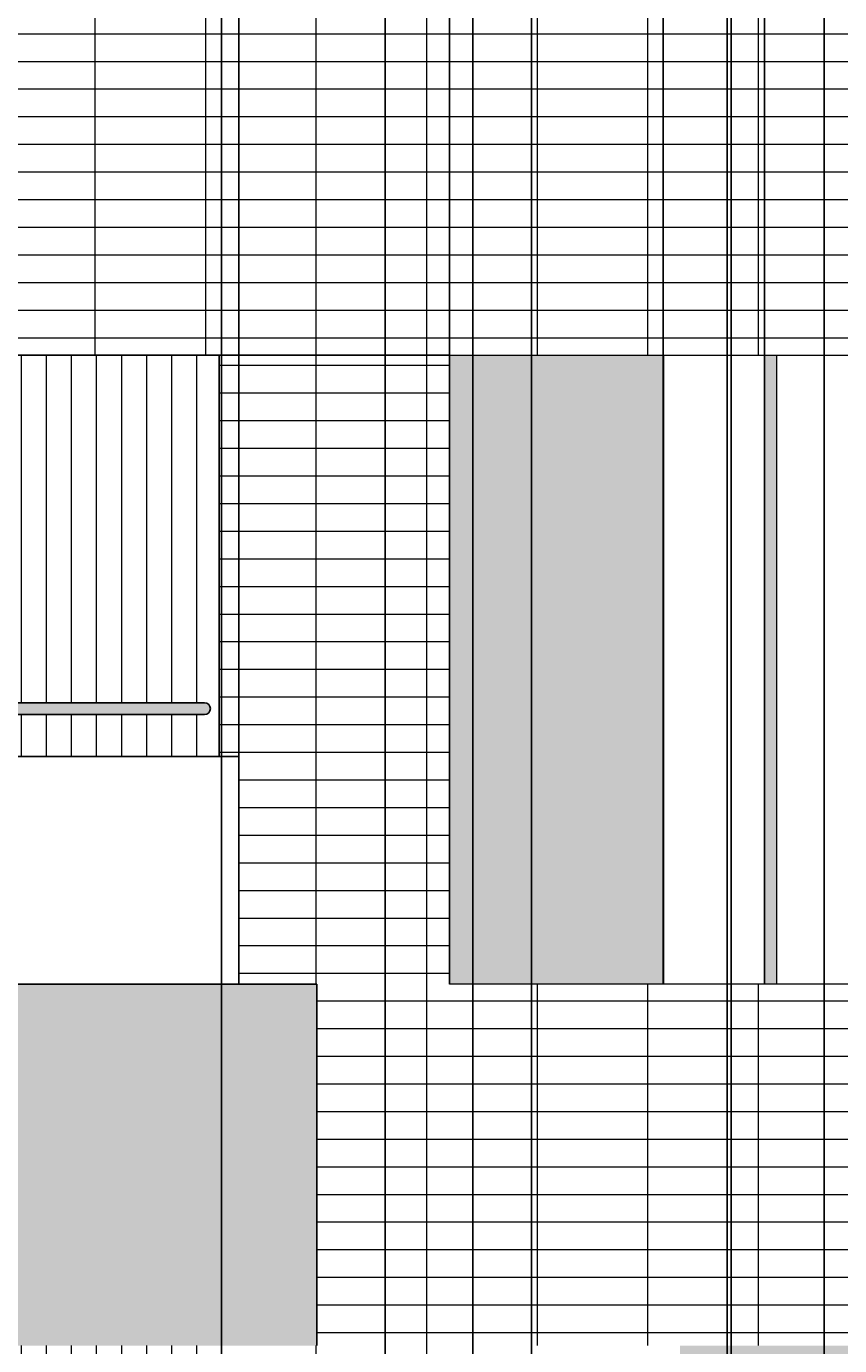
# Model space of a CAD drawing. Units: inches. Extents: x 241 to 943, y 109 to 1396.
# Tile 26 of 34: x 532 to 670, y 842 to 1065. Entities that reach past the tile are written whole.
import ezdxf

# ---------------------------------------------------------------- set-up
doc = ezdxf.new("R2010")
doc.units = ezdxf.units.IN
doc.header["$MEASUREMENT"] = 0
for name, color, linetype, lineweight in [('A-ANNO-DIMS', 2, 'Continuous', 18), ('A-ELEV', 7, 'Continuous', 25), ('A-ELEV-SHAD', 9, 'Continuous', 13), ('A-GLAZ', 4, 'Continuous', 18), ('A-GLAZ-PATT', 18, 'Continuous', 13), ('A-WALL-PATT', 8, 'Continuous', 13)]:
    doc.layers.add(name, color=color, linetype=linetype, lineweight=lineweight)
doc.styles.get("Standard").update_dxf_attribs({"font": 'arial.ttf'})
doc.dimstyles.get("Standard").update_dxf_attribs({"dimtxt": 1.4375, "dimasz": 0.18, "dimexe": 0.18, "dimexo": 0.0625, "dimgap": 0.09, "dimtad": 0, "dimtih": 1, "dimtoh": 1, "dimdec": 4, "dimzin": 0, "dimdsep": 46, "dimlunit": 4, "dimtxsty": 'Standard', "dimcen": 0.09, "dimadec": 0, "dimazin": 0, "dimtfac": 1, "dimtdec": 4, "dimtofl": 0, "dimtmove": 0, "dimatfit": 3, "dimfxl": 1, "dimtolj": 1, "dimtzin": 0, "dimarcsym": 0})

# ---------------------------------------------------------------- blocks, each defined once
blk = doc.blocks.new('*D12')
at = {"layer": 'A-ANNO-DIMS', "color": 0, "lineweight": -2, "transparency": 16777216}
for p, q in [((530.23, 384.24), (530.23, 1395.05)), ((530.41, 1394.87), (587.56, 1394.87)), ((650.73, 1394.87), (593.58, 1394.87)), ((650.91, 384.24), (650.91, 1395.05))]:
    blk.add_line(p, q, dxfattribs=at)
at = {"layer": 'A-ANNO-DIMS', "color": 0, "transparency": 16777216}
for points in [[(530.41, 1394.9), (530.41, 1394.84), (530.23, 1394.87)], [(650.73, 1394.9), (650.73, 1394.84), (650.91, 1394.87)]]:
    blk.add_solid(points, dxfattribs=at)
at = {"layer": 'Defpoints', "color": 0, "transparency": 16777216}
for p in [(650.91, 1394.87), (530.23, 384.18), (650.91, 384.18)]:
    blk.add_point(p, dxfattribs=at)
at = {"layer": 'A-ANNO-DIMS', "color": 0, "transparency": 16777216, "insert": (590.57, 1394.87), "char_height": 1.438, "attachment_point": 5}
blk.add_mtext('\\A1;120.68', dxfattribs=at)
blk = doc.blocks.new('*D13')
at = {"layer": 'A-ANNO-DIMS', "color": 0, "lineweight": -2, "transparency": 16777216}
for p, q in [((650.91, 384.24), (650.91, 1395.05)), ((651.09, 1394.87), (656.14, 1394.87)), ((667.21, 1394.87), (662.16, 1394.87)), ((667.39, 290.06), (667.39, 1395.05))]:
    blk.add_line(p, q, dxfattribs=at)
at = {"layer": 'A-ANNO-DIMS', "color": 0, "transparency": 16777216}
for points in [[(651.09, 1394.9), (651.09, 1394.84), (650.91, 1394.87)], [(667.21, 1394.9), (667.21, 1394.84), (667.39, 1394.87)]]:
    blk.add_solid(points, dxfattribs=at)
at = {"layer": 'Defpoints', "color": 0, "transparency": 16777216}
for p in [(667.39, 1394.87), (650.91, 384.18), (667.39, 290)]:
    blk.add_point(p, dxfattribs=at)
at = {"layer": 'A-ANNO-DIMS', "color": 0, "transparency": 16777216, "insert": (659.15, 1394.87), "char_height": 1.438, "attachment_point": 5}
blk.add_mtext('\\A1;16.486', dxfattribs=at)
blk = doc.blocks.new('*D14')
at = {"layer": 'A-ANNO-DIMS', "color": 0, "lineweight": -2, "transparency": 16777216}
for p, q in [((667.39, 290.06), (667.39, 1395.05)), ((667.57, 1394.87), (727.7, 1394.87)), ((793.85, 1394.87), (733.72, 1394.87)), ((794.03, 290.06), (794.03, 1395.05))]:
    blk.add_line(p, q, dxfattribs=at)
at = {"layer": 'A-ANNO-DIMS', "color": 0, "transparency": 16777216}
for points in [[(667.57, 1394.9), (667.57, 1394.84), (667.39, 1394.87)], [(793.85, 1394.9), (793.85, 1394.84), (794.03, 1394.87)]]:
    blk.add_solid(points, dxfattribs=at)
at = {"layer": 'Defpoints', "color": 0, "transparency": 16777216}
for p in [(794.03, 1394.87), (667.39, 290), (794.03, 290)]:
    blk.add_point(p, dxfattribs=at)
at = {"layer": 'A-ANNO-DIMS', "color": 0, "transparency": 16777216, "insert": (730.71, 1394.87), "char_height": 1.438, "attachment_point": 5}
blk.add_mtext('\\A1;126.63', dxfattribs=at)
blk = doc.blocks.new('*D62')
at = {"layer": 'A-ANNO-DIMS', "color": 0, "lineweight": -2, "transparency": 16777216}
for p, q in [((424.11, 568.89), (424.11, 1395.05)), ((424.29, 1394.87), (492.35, 1394.87)), ((565.02, 1394.87), (496.96, 1394.87)), ((565.2, 568.89), (565.2, 1395.05))]:
    blk.add_line(p, q, dxfattribs=at)
at = {"layer": 'A-ANNO-DIMS', "color": 0, "transparency": 16777216}
for points in [[(424.29, 1394.9), (424.29, 1394.84), (424.11, 1394.87)], [(565.02, 1394.9), (565.02, 1394.84), (565.2, 1394.87)]]:
    blk.add_solid(points, dxfattribs=at)
at = {"layer": 'Defpoints', "color": 0, "transparency": 16777216}
for p in [(565.2, 1394.87), (424.11, 568.83), (565.2, 568.83)]:
    blk.add_point(p, dxfattribs=at)
at = {"layer": 'A-ANNO-DIMS', "color": 0, "transparency": 16777216, "insert": (494.66, 1394.87), "char_height": 1.438, "attachment_point": 5}
blk.add_mtext('\\A1;141.1', dxfattribs=at)
blk = doc.blocks.new('*D63')
at = {"layer": 'A-ANNO-DIMS', "color": 0, "lineweight": -2, "transparency": 16777216}
for p, q in [((651.6, 568.89), (651.6, 1395.05)), ((651.78, 1394.87), (719.84, 1394.87)), ((792.51, 1394.87), (724.45, 1394.87)), ((792.69, 568.89), (792.69, 1395.05))]:
    blk.add_line(p, q, dxfattribs=at)
at = {"layer": 'A-ANNO-DIMS', "color": 0, "transparency": 16777216}
for points in [[(651.78, 1394.9), (651.78, 1394.84), (651.6, 1394.87)], [(792.51, 1394.9), (792.51, 1394.84), (792.69, 1394.87)]]:
    blk.add_solid(points, dxfattribs=at)
at = {"layer": 'Defpoints', "color": 0, "transparency": 16777216}
for p in [(792.69, 1394.87), (651.6, 568.83), (792.69, 568.83)]:
    blk.add_point(p, dxfattribs=at)
at = {"layer": 'A-ANNO-DIMS', "color": 0, "transparency": 16777216, "insert": (722.14, 1394.87), "char_height": 1.438, "attachment_point": 5}
blk.add_mtext('\\A1;141.1', dxfattribs=at)
blk = doc.blocks.new('*D65')
at = {"layer": 'A-ANNO-DIMS', "color": 0, "lineweight": -2, "transparency": 16777216}
for p, q in [((424.11, 700.85), (424.11, 1395.05)), ((424.29, 1394.87), (505.52, 1394.87)), ((592.77, 1394.87), (511.54, 1394.87)), ((592.95, 700.85), (592.95, 1395.05))]:
    blk.add_line(p, q, dxfattribs=at)
at = {"layer": 'A-ANNO-DIMS', "color": 0, "transparency": 16777216}
for points in [[(424.29, 1394.9), (424.29, 1394.84), (424.11, 1394.87)], [(592.77, 1394.9), (592.77, 1394.84), (592.95, 1394.87)]]:
    blk.add_solid(points, dxfattribs=at)
at = {"layer": 'Defpoints', "color": 0, "transparency": 16777216}
for p in [(592.95, 1394.87), (424.11, 700.79), (592.95, 700.79)]:
    blk.add_point(p, dxfattribs=at)
at = {"layer": 'A-ANNO-DIMS', "color": 0, "transparency": 16777216, "insert": (508.53, 1394.87), "char_height": 1.438, "attachment_point": 5}
blk.add_mtext('\\A1;168.85', dxfattribs=at)
blk = doc.blocks.new('*D66')
at = {"layer": 'A-ANNO-DIMS', "color": 0, "lineweight": -2, "transparency": 16777216}
for p, q in [((617.76, 702.85), (617.76, 1395.05)), ((617.94, 1394.87), (680.69, 1394.87)), ((749.45, 1394.87), (686.7, 1394.87)), ((749.63, 702.85), (749.63, 1395.05))]:
    blk.add_line(p, q, dxfattribs=at)
at = {"layer": 'A-ANNO-DIMS', "color": 0, "transparency": 16777216}
for points in [[(617.94, 1394.9), (617.94, 1394.84), (617.76, 1394.87)], [(749.45, 1394.9), (749.45, 1394.84), (749.63, 1394.87)]]:
    blk.add_solid(points, dxfattribs=at)
at = {"layer": 'Defpoints', "color": 0, "transparency": 16777216}
for p in [(749.63, 1394.87), (617.76, 702.79), (749.63, 702.79)]:
    blk.add_point(p, dxfattribs=at)
at = {"layer": 'A-ANNO-DIMS', "color": 0, "transparency": 16777216, "insert": (683.7, 1394.87), "char_height": 1.438, "attachment_point": 5}
blk.add_mtext('\\A1;131.87', dxfattribs=at)
blk = doc.blocks.new('*D67')
at = {"layer": 'A-ANNO-DIMS', "color": 0, "lineweight": -2, "transparency": 16777216}
for p, q in [((389.04, 773.55), (389.04, 1395.05)), ((389.22, 1394.87), (495.34, 1394.87)), ((607.64, 1394.87), (501.52, 1394.87)), ((607.82, 773.55), (607.82, 1395.05))]:
    blk.add_line(p, q, dxfattribs=at)
at = {"layer": 'A-ANNO-DIMS', "color": 0, "transparency": 16777216}
for points in [[(389.22, 1394.9), (389.22, 1394.84), (389.04, 1394.87)], [(607.64, 1394.9), (607.64, 1394.84), (607.82, 1394.87)]]:
    blk.add_solid(points, dxfattribs=at)
at = {"layer": 'Defpoints', "color": 0, "transparency": 16777216}
for p in [(607.82, 1394.87), (389.04, 773.49), (607.82, 773.49)]:
    blk.add_point(p, dxfattribs=at)
at = {"layer": 'A-ANNO-DIMS', "color": 0, "transparency": 16777216, "insert": (498.43, 1394.87), "char_height": 1.438, "attachment_point": 5}
blk.add_mtext('\\A1;218.77', dxfattribs=at)
blk = doc.blocks.new('*D68')
at = {"layer": 'A-ANNO-DIMS', "color": 0, "lineweight": -2, "transparency": 16777216}
for p, q in [((617.76, 841.6), (617.76, 1395.05)), ((617.94, 1394.87), (702.22, 1394.87)), ((792.51, 1394.87), (708.23, 1394.87)), ((792.69, 841.6), (792.69, 1395.05))]:
    blk.add_line(p, q, dxfattribs=at)
at = {"layer": 'A-ANNO-DIMS', "color": 0, "transparency": 16777216}
for points in [[(617.94, 1394.9), (617.94, 1394.84), (617.76, 1394.87)], [(792.51, 1394.9), (792.51, 1394.84), (792.69, 1394.87)]]:
    blk.add_solid(points, dxfattribs=at)
at = {"layer": 'Defpoints', "color": 0, "transparency": 16777216}
for p in [(792.69, 1394.87), (617.76, 841.54), (792.69, 841.54)]:
    blk.add_point(p, dxfattribs=at)
at = {"layer": 'A-ANNO-DIMS', "color": 0, "transparency": 16777216, "insert": (705.23, 1394.87), "char_height": 1.438, "attachment_point": 5}
blk.add_mtext('\\A1;174.93', dxfattribs=at)
blk = doc.blocks.new('*D69')
at = {"layer": 'A-ANNO-DIMS', "color": 0, "lineweight": -2, "transparency": 16777216}
for p, q in [((389.04, 941.55), (389.04, 1395.05)), ((389.22, 1394.87), (476.28, 1394.87)), ((567.95, 1394.87), (480.9, 1394.87)), ((568.13, 941.55), (568.13, 1395.05))]:
    blk.add_line(p, q, dxfattribs=at)
at = {"layer": 'A-ANNO-DIMS', "color": 0, "transparency": 16777216}
for points in [[(389.22, 1394.9), (389.22, 1394.84), (389.04, 1394.87)], [(567.95, 1394.9), (567.95, 1394.84), (568.13, 1394.87)]]:
    blk.add_solid(points, dxfattribs=at)
at = {"layer": 'Defpoints', "color": 0, "transparency": 16777216}
for p in [(568.13, 1394.87), (389.04, 941.49), (568.13, 941.49)]:
    blk.add_point(p, dxfattribs=at)
at = {"layer": 'A-ANNO-DIMS', "color": 0, "transparency": 16777216, "insert": (478.59, 1394.87), "char_height": 1.438, "attachment_point": 5}
blk.add_mtext('\\A1;179.1', dxfattribs=at)
blk = doc.blocks.new('*D70')
at = {"layer": 'A-ANNO-DIMS', "color": 0, "lineweight": -2, "transparency": 16777216}
for p, q in [((603.87, 1009.6), (603.87, 1395.05)), ((604.05, 1394.87), (674.69, 1394.87)), ((751.33, 1394.87), (680.69, 1394.87)), ((751.51, 1009.6), (751.51, 1395.05))]:
    blk.add_line(p, q, dxfattribs=at)
at = {"layer": 'A-ANNO-DIMS', "color": 0, "transparency": 16777216}
for points in [[(604.05, 1394.9), (604.05, 1394.84), (603.87, 1394.87)], [(751.33, 1394.9), (751.33, 1394.84), (751.51, 1394.87)]]:
    blk.add_solid(points, dxfattribs=at)
at = {"layer": 'Defpoints', "color": 0, "transparency": 16777216}
for p in [(751.51, 1394.87), (603.87, 1009.54), (751.51, 1009.54)]:
    blk.add_point(p, dxfattribs=at)
at = {"layer": 'A-ANNO-DIMS', "color": 0, "transparency": 16777216, "insert": (677.69, 1394.87), "char_height": 1.438, "attachment_point": 5}
blk.add_mtext('\\A1;147.64', dxfattribs=at)
blk = doc.blocks.new('*D82')
at = {"layer": 'A-ANNO-DIMS', "color": 0, "lineweight": -2, "transparency": 16777216}
for p, q in [((565.2, 568.89), (565.2, 1395.05)), ((565.38, 1394.87), (605.89, 1394.87)), ((651.42, 1394.87), (610.91, 1394.87)), ((651.6, 568.89), (651.6, 1395.05))]:
    blk.add_line(p, q, dxfattribs=at)
at = {"layer": 'A-ANNO-DIMS', "color": 0, "transparency": 16777216}
for points in [[(565.38, 1394.9), (565.38, 1394.84), (565.2, 1394.87)], [(651.42, 1394.9), (651.42, 1394.84), (651.6, 1394.87)]]:
    blk.add_solid(points, dxfattribs=at)
at = {"layer": 'Defpoints', "color": 0, "transparency": 16777216}
for p in [(651.6, 1394.87), (565.2, 568.83), (651.6, 568.83)]:
    blk.add_point(p, dxfattribs=at)
at = {"layer": 'A-ANNO-DIMS', "color": 0, "transparency": 16777216, "insert": (608.4, 1394.87), "char_height": 1.438, "attachment_point": 5}
blk.add_mtext('\\A1;86.40', dxfattribs=at)
blk = doc.blocks.new('*D83')
at = {"layer": 'A-ANNO-DIMS', "color": 0, "lineweight": -2, "transparency": 16777216}
for p, q in [((592.95, 700.85), (592.95, 1395.05)), ((593.13, 1394.87), (602.27, 1394.87)), ((617.58, 1394.87), (608.45, 1394.87)), ((617.76, 702.85), (617.76, 1395.05))]:
    blk.add_line(p, q, dxfattribs=at)
at = {"layer": 'A-ANNO-DIMS', "color": 0, "transparency": 16777216}
for points in [[(593.13, 1394.9), (593.13, 1394.84), (592.95, 1394.87)], [(617.58, 1394.9), (617.58, 1394.84), (617.76, 1394.87)]]:
    blk.add_solid(points, dxfattribs=at)
at = {"layer": 'Defpoints', "color": 0, "transparency": 16777216}
for p in [(617.76, 1394.87), (617.76, 702.79), (592.95, 700.79)]:
    blk.add_point(p, dxfattribs=at)
at = {"layer": 'A-ANNO-DIMS', "color": 0, "transparency": 16777216, "insert": (605.36, 1394.87), "char_height": 1.438, "attachment_point": 5}
blk.add_mtext('\\A1;24.805', dxfattribs=at)
blk = doc.blocks.new('*D89')
at = {"layer": 'A-ANNO-DIMS', "color": 0, "lineweight": -2, "transparency": 16777216}
for p, q in [((377.04, 841.6), (377.04, 1395.05)), ((377.22, 1394.87), (494.32, 1394.87)), ((617.58, 1394.87), (500.48, 1394.87)), ((617.76, 841.6), (617.76, 1395.05))]:
    blk.add_line(p, q, dxfattribs=at)
at = {"layer": 'A-ANNO-DIMS', "color": 0, "transparency": 16777216}
for points in [[(377.22, 1394.9), (377.22, 1394.84), (377.04, 1394.87)], [(617.58, 1394.9), (617.58, 1394.84), (617.76, 1394.87)]]:
    blk.add_solid(points, dxfattribs=at)
at = {"layer": 'Defpoints', "color": 0, "transparency": 16777216}
for p in [(617.76, 1394.87), (377.04, 841.54), (617.76, 841.54)]:
    blk.add_point(p, dxfattribs=at)
at = {"layer": 'A-ANNO-DIMS', "color": 0, "transparency": 16777216, "insert": (497.4, 1394.87), "char_height": 1.438, "attachment_point": 5}
blk.add_mtext('\\A1;240.72', dxfattribs=at)
blk = doc.blocks.new('*D90')
at = {"layer": 'A-ANNO-DIMS', "color": 0, "lineweight": -2, "transparency": 16777216}
for p, q in [((568.13, 941.55), (568.13, 1395.05)), ((568.31, 1394.87), (582.92, 1394.87)), ((603.69, 1394.87), (589.08, 1394.87)), ((603.87, 902.92), (603.87, 1395.05))]:
    blk.add_line(p, q, dxfattribs=at)
at = {"layer": 'A-ANNO-DIMS', "color": 0, "transparency": 16777216}
for points in [[(568.31, 1394.9), (568.31, 1394.84), (568.13, 1394.87)], [(603.69, 1394.9), (603.69, 1394.84), (603.87, 1394.87)]]:
    blk.add_solid(points, dxfattribs=at)
at = {"layer": 'Defpoints', "color": 0, "transparency": 16777216}
for p in [(603.87, 1394.87), (568.13, 941.49), (603.87, 902.85)]:
    blk.add_point(p, dxfattribs=at)
at = {"layer": 'A-ANNO-DIMS', "color": 0, "transparency": 16777216, "insert": (586, 1394.87), "char_height": 1.438, "attachment_point": 5}
blk.add_mtext('\\A1;35.735', dxfattribs=at)
blk = doc.blocks.new('*D99')
at = {"layer": 'A-ANNO-DIMS', "color": 0, "lineweight": -2, "transparency": 16777216}
for p, q in [((417.09, 181.71), (417.09, 1395.05)), ((417.27, 1394.87), (539.16, 1394.87)), ((667.21, 1394.87), (545.33, 1394.87)), ((667.39, 214.58), (667.39, 1395.05))]:
    blk.add_line(p, q, dxfattribs=at)
at = {"layer": 'A-ANNO-DIMS', "color": 0, "transparency": 16777216}
for points in [[(417.27, 1394.9), (417.27, 1394.84), (417.09, 1394.87)], [(667.21, 1394.9), (667.21, 1394.84), (667.39, 1394.87)]]:
    blk.add_solid(points, dxfattribs=at)
at = {"layer": 'Defpoints', "color": 0, "transparency": 16777216}
for p in [(667.39, 1394.87), (667.39, 214.52), (417.09, 181.65)]:
    blk.add_point(p, dxfattribs=at)
at = {"layer": 'A-ANNO-DIMS', "color": 0, "transparency": 16777216, "insert": (542.24, 1394.87), "char_height": 1.438, "attachment_point": 5}
blk.add_mtext('\\A1;250.30', dxfattribs=at)
blk = doc.blocks.new('*D113')
at = {"layer": 'A-ANNO-DIMS', "color": 0, "lineweight": -2, "transparency": 16777216}
for p, q in [((603.87, 902.92), (603.87, 1395.05)), ((604.05, 1394.87), (618.91, 1394.87)), ((639.93, 1394.87), (625.07, 1394.87)), ((640.11, 902.92), (640.11, 1395.05))]:
    blk.add_line(p, q, dxfattribs=at)
at = {"layer": 'A-ANNO-DIMS', "color": 0, "transparency": 16777216}
for points in [[(604.05, 1394.9), (604.05, 1394.84), (603.87, 1394.87)], [(639.93, 1394.9), (639.93, 1394.84), (640.11, 1394.87)]]:
    blk.add_solid(points, dxfattribs=at)
at = {"layer": 'Defpoints', "color": 0, "transparency": 16777216}
for p in [(640.11, 1394.87), (603.87, 902.85), (640.11, 902.85)]:
    blk.add_point(p, dxfattribs=at)
at = {"layer": 'A-ANNO-DIMS', "color": 0, "transparency": 16777216, "insert": (621.99, 1394.87), "char_height": 1.438, "attachment_point": 5}
blk.add_mtext('\\A1;36.245', dxfattribs=at)
blk = doc.blocks.new('*D114')
at = {"layer": 'A-ANNO-DIMS', "color": 0, "lineweight": -2, "transparency": 16777216}
for p, q in [((640.11, 902.92), (640.11, 1395.05)), ((640.29, 1394.87), (646.25, 1394.87)), ((657.11, 1394.87), (651.15, 1394.87)), ((657.29, 902.92), (657.29, 1395.05))]:
    blk.add_line(p, q, dxfattribs=at)
at = {"layer": 'A-ANNO-DIMS', "color": 0, "transparency": 16777216}
for points in [[(640.29, 1394.9), (640.29, 1394.84), (640.11, 1394.87)], [(657.11, 1394.9), (657.11, 1394.84), (657.29, 1394.87)]]:
    blk.add_solid(points, dxfattribs=at)
at = {"layer": 'Defpoints', "color": 0, "transparency": 16777216}
for p in [(657.29, 1394.87), (640.11, 902.85), (657.29, 902.85)]:
    blk.add_point(p, dxfattribs=at)
at = {"layer": 'A-ANNO-DIMS', "color": 0, "transparency": 16777216, "insert": (648.7, 1394.87), "char_height": 1.438, "attachment_point": 5}
blk.add_mtext('\\A1;17.18', dxfattribs=at)
blk = doc.blocks.new('*D115')
at = {"layer": 'A-ANNO-DIMS', "color": 0, "lineweight": -2, "transparency": 16777216}
for p, q in [((657.29, 902.92), (657.29, 1395.05)), ((657.47, 1394.87), (664.4, 1394.87)), ((677.51, 1394.87), (670.58, 1394.87)), ((677.69, 902.92), (677.69, 1395.05))]:
    blk.add_line(p, q, dxfattribs=at)
at = {"layer": 'A-ANNO-DIMS', "color": 0, "transparency": 16777216}
for points in [[(657.47, 1394.9), (657.47, 1394.84), (657.29, 1394.87)], [(677.51, 1394.9), (677.51, 1394.84), (677.69, 1394.87)]]:
    blk.add_solid(points, dxfattribs=at)
at = {"layer": 'Defpoints', "color": 0, "transparency": 16777216}
for p in [(677.69, 1394.87), (657.29, 902.85), (677.69, 902.85)]:
    blk.add_point(p, dxfattribs=at)
at = {"layer": 'A-ANNO-DIMS', "color": 0, "transparency": 16777216, "insert": (667.49, 1394.87), "char_height": 1.438, "attachment_point": 5}
blk.add_mtext('\\A1;20.396', dxfattribs=at)

msp = doc.modelspace()

# ---------------------------------------------------------------- hatches: boundary and pattern name
at = {"layer": 'A-ELEV-SHAD'}
h = msp.add_hatch(color=256, dxfattribs=at)
h.dxf.hatch_style = 1
h.paths.add_polyline_path([(508.3064, 1070.8538), (377.0391, 1070.8538), (377.0391, 1009.5382), (508.3064, 1009.5382)])
h.paths.add_polyline_path([(508.3064, 1238.8538), (377.0391, 1238.8538), (377.0391, 1177.5382), (508.3064, 1177.5382)])
h.paths.add_polyline_path([(581.3632, 902.8538), (568.1348, 902.8538), (553.5166, 902.8538), (377.0391, 902.8538), (377.0391, 841.5382), (553.5166, 841.5382), (564.8076, 841.5382), (581.3632, 841.5382)])
h.paths.add_polyline_path([(820.8374, 1275.9142), (747.7579, 1275.9142), (747.7579, 1238.8538), (820.8374, 1238.8538)])
h.paths.add_polyline_path([(820.8374, 1238.8538), (747.7579, 1238.8538), (747.9341, 1223.0633), (820.8374, 1223.0633)])
h.paths.add_polyline_path([(396.3125, 841.5382), (377.0391, 841.5382), (377.0391, 734.8538), (389.0429, 734.8538), (389.0429, 735.188), (389.0429, 773.4916), (396.3125, 773.4916), (396.3125, 780.5808), (390.5597, 780.5808), (388.0428, 780.5808, -1), (388.0428, 782.5808), (390.5597, 782.5808), (396.3125, 782.5808)])
h = msp.add_hatch(color=256, dxfattribs=at)
h.dxf.hatch_style = 1
h.paths.add_polyline_path([(537.4269, 698.7912), (534.1778, 698.7912), (534.1778, 659.3434), (537.4269, 659.3434)])
h.paths.add_polyline_path([(508.0803, 698.7912), (450.9259, 698.7912), (450.9259, 659.3434), (452.9259, 659.3434), (452.9259, 696.7912), (506.0803, 696.7912), (506.0803, 659.3434), (508.0803, 659.3434)])
h.paths.add_polyline_path([(481.5031, 696.7912), (479.5031, 696.7912), (479.5031, 659.3434), (481.5031, 659.3434)], flags=17)
h.paths.add_polyline_path([(481.5031, 657.3434), (479.5031, 657.3434), (479.5031, 653.3371), (481.5031, 653.3371)], flags=17)
h.paths.add_polyline_path([(508.0803, 657.3434), (506.0803, 657.3434), (506.0803, 653.3371), (452.9259, 653.3371), (452.9259, 657.3434), (450.9259, 657.3434), (450.9259, 651.3371), (508.0803, 651.3371)])
h.paths.add_polyline_path([(428.1173, 839.5382), (426.1173, 839.5382), (426.1173, 786.9154), (428.1173, 786.9154)], flags=17)
h.paths.add_polyline_path([(470.8692, 839.5382), (468.8692, 839.5382), (468.8692, 786.9154), (470.8692, 786.9154)], flags=17)
h.paths.add_polyline_path([(508.3064, 841.5382), (396.3125, 841.5382), (396.3125, 782.5808), (398.3125, 782.5808), (398.3125, 839.5382), (506.3064, 839.5382), (506.3064, 782.5808), (508.3064, 782.5808)])
h.paths.add_polyline_path([(398.3125, 780.5808), (396.3125, 780.5808), (396.3125, 773.4916), (398.3125, 773.4916)])
h.paths.add_polyline_path([(508.3064, 780.5808), (506.3064, 780.5808), (506.3064, 773.4916), (508.3064, 773.4916)])
h.paths.add_polyline_path([(715.6236, 841.5382), (678.2674, 841.5382), (678.2674, 734.8538), (715.6236, 734.8538)])
h.paths.add_polyline_path([(680.2674, 839.5382), (682.4526, 839.5382), (713.6236, 839.5382), (713.6236, 736.9235), (690.2047, 736.9235), (680.2674, 736.9235)], flags=16)
h.paths.add_polyline_path([(792.691, 841.5382), (747.7579, 841.5382), (747.7579, 734.8538), (754.5373, 734.8538), (754.5373, 736.9235), (754.5373, 839.5382), (756.7224, 839.5382), (787.8934, 839.5382), (787.8934, 765.9585), (792.691, 765.9585)])
h.paths.add_polyline_path([(659.2925, 1009.5382), (657.2925, 1009.5382), (657.2925, 902.8538), (659.2925, 902.8538)])
h.paths.add_polyline_path([(751.5078, 976.6275), (712.5839, 976.6275), (712.5839, 974.6275), (751.5078, 974.6275)])
h.paths.add_polyline_path([(470.8692, 1007.5382), (468.8692, 1007.5382), (468.8692, 954.9154), (470.8692, 954.9154)], flags=17)
h.paths.add_polyline_path([(508.3064, 1009.5382), (396.3125, 1009.5382), (396.3125, 950.5808), (398.3125, 950.5808), (398.3125, 1007.5382), (506.3064, 1007.5382), (506.3064, 950.5808), (508.3064, 950.5808)])
h.paths.add_polyline_path([(428.1173, 1007.5382), (426.1173, 1007.5382), (426.1173, 954.9154), (428.1173, 954.9154)], flags=17)
h.paths.add_polyline_path([(398.3125, 948.5808), (396.3125, 948.5808), (396.3125, 941.4916), (398.3125, 941.4916)])
h.paths.add_polyline_path([(508.3064, 948.5808), (506.3064, 948.5808), (506.3064, 941.4916), (508.3064, 941.4916)])
h.paths.add_polyline_path([(428.1173, 1175.5382), (426.1173, 1175.5382), (426.1173, 1122.9154), (428.1173, 1122.9154)], flags=17)
h.paths.add_polyline_path([(508.3064, 1177.5382), (396.3125, 1177.5382), (396.3125, 1118.5808), (398.3125, 1118.5808), (398.3125, 1175.5382), (506.3064, 1175.5382), (506.3064, 1118.5808), (506.8039, 1118.5808, -1), (506.8039, 1116.5808), (506.3064, 1116.5808), (506.3064, 1109.4916), (508.3064, 1109.4916)])
h.paths.add_polyline_path([(470.8692, 1175.5382), (468.8692, 1175.5382), (468.8692, 1122.9154), (470.8692, 1122.9154)], flags=17)
h.paths.add_polyline_path([(398.3125, 1116.5808), (396.3125, 1116.5808), (396.3125, 1109.4916), (398.3125, 1109.4916)], flags=17)
h.paths.add_polyline_path([(724.819, 1177.7336), (533.952, 1177.7336), (533.952, 1108.1686), (724.819, 1108.1686)])
h.paths.add_polyline_path([(535.952, 1175.7336), (722.819, 1175.7336), (722.819, 1110.1686), (535.952, 1110.1686)], flags=0)
h.paths.add_polyline_path([(622.521, 1136.0739), (643.4534, 1136.0739), (643.4534, 1134.0739), (622.521, 1134.0739)], flags=0)
h.paths.add_polyline_path([(722.819, 1175.7336), (535.952, 1175.7336), (535.952, 1110.1686), (722.819, 1110.1686)], flags=16)
h.paths.add_polyline_path([(565.947, 1151.5772), (535.952, 1151.5772), (535.952, 1149.5772), (565.947, 1149.5772)], flags=0)
at = {"layer": 'A-GLAZ-PATT'}
h = msp.add_hatch(dxfattribs=at)
h.set_pattern_fill('GOST_GLASS', color=256, scale=0.89)
h.set_pattern_definition([(45, (0, 0), (7.5519, 0), [4.45, -6.23]), (45, (1.888, 0), (7.5519, 0), [1.78, -8.9]), (45, (0, 1.888), (7.5519, 0), [1.78, -8.9])])
h.paths.add_polyline_path([(676.8698, 700.7912), (652.0129, 700.7912), (652.0129, 628.4013), (676.8698, 628.4013)])
h.paths.add_polyline_path([(650.0129, 700.7912), (617.7594, 700.7912), (617.7594, 628.4013), (650.0129, 628.4013)])
h.paths.add_polyline_path([(747.7579, 841.5382), (715.6236, 841.5382), (715.6236, 734.8538), (747.7579, 734.8538)])
h.paths.add_polyline_path([(678.2674, 841.5382), (642.9197, 841.5382), (642.9197, 734.8538), (678.2674, 734.8538)])
h.paths.add_polyline_path([(712.5839, 1009.5382), (677.6886, 1009.5382), (677.6886, 902.8538), (712.5839, 902.8538)])
h.paths.add_polyline_path([(640.1141, 1009.5382), (603.8694, 1009.5382), (603.8694, 902.8538), (640.1141, 902.8538)])
h.paths.add_polyline_path([(682.8748, 1175.7336), (643.4534, 1175.7336), (643.4534, 1110.1686), (682.8748, 1110.1686)])
h.paths.add_polyline_path([(602.3616, 1175.7336), (565.947, 1175.7336), (565.947, 1110.1686), (602.3616, 1110.1686)])
h = msp.add_hatch(dxfattribs=at)
h.set_pattern_fill('ANSI31', color=256, scale=34, angle=45)
h.paths.add_polyline_path([(486.3418, 786.9154), (413.1187, 786.9154), (413.1187, 761.2284), (486.3418, 761.2284)])
h.paths.add_polyline_path([(486.3418, 954.9154), (413.1187, 954.9154), (413.1187, 929.2284), (486.3418, 929.2284)])
h.paths.add_polyline_path([(462.1074, 289.6933), (390.895, 289.6933), (390.895, 277.4626), (390.895, 274.3507), (462.1074, 274.3507), (462.1074, 277.4626)])
h.paths.add_polyline_path([(500.3323, 289.6933), (479.596, 289.6933), (479.596, 274.3507), (500.3323, 274.3507)])
h.paths.add_polyline_path([(450.9259, 566.8295), (426.1086, 566.8295), (426.1086, 498.4395), (446.4348, 498.4395), (446.4348, 519.3754), (450.9259, 519.3754), (450.9259, 525.3816), (445.5808, 525.3816, -1), (445.5808, 527.3816), (450.9259, 527.3816)])
h.paths.add_polyline_path([(563.2023, 508.9074), (534.1778, 508.9074), (508.1906, 508.9074), (508.1906, 498.4395), (563.2023, 498.4395)])
h.paths.add_polyline_path([(747.6328, 700.7912), (712.0171, 700.7912), (712.0171, 628.4013), (747.6328, 628.4013)])
h.paths.add_polyline_path([(446.4348, 643.7483), (426.1086, 643.7483), (426.1086, 630.4013), (446.4348, 630.4013)])
h.paths.add_polyline_path([(564.8076, 841.5382), (553.5166, 841.5382), (508.3064, 841.5382), (508.3064, 782.5808), (564.8076, 782.5808)])
h.paths.add_polyline_path([(564.8076, 780.5808), (508.3064, 780.5808), (508.3064, 773.4916), (564.8076, 773.4916)])
h.paths.add_polyline_path([(792.691, 762.5799), (759.6248, 762.5799), (759.6248, 736.9235), (759.6248, 734.8538), (792.691, 734.8538)])
h.paths.add_polyline_path([(564.8076, 1009.5382), (553.5166, 1009.5382), (508.3064, 1009.5382), (508.3064, 950.5808), (562.3033, 950.5808, -1), (562.3033, 948.5808), (508.3064, 948.5808), (508.3064, 941.4916), (564.8076, 941.4916)])
h.paths.add_polyline_path([(486.3418, 1122.9154), (413.1187, 1122.9154), (413.1187, 1097.2284), (486.3418, 1097.2284)])
h = msp.add_hatch(color=256, dxfattribs=at)
h.dxf.hatch_style = 1
h.paths.add_polyline_path([(396.3125, 1118.5808), (390.5597, 1118.5808), (388.0428, 1118.5808, 1), (388.0428, 1116.5808), (390.5597, 1116.5808), (396.3125, 1116.5808)])
h.paths.add_polyline_path([(398.3125, 1118.5808), (396.3125, 1118.5808), (396.3125, 1116.5808), (398.3125, 1116.5808)])
h.paths.add_polyline_path([(413.1187, 1118.5808), (398.3125, 1118.5808), (398.3125, 1116.5808), (413.1187, 1116.5808)])
h.paths.add_polyline_path([(506.3064, 1118.5808), (486.3418, 1118.5808), (486.3418, 1116.5808), (506.3064, 1116.5808)])
h.paths.add_polyline_path([(506.8039, 1118.5808), (506.3064, 1118.5808), (506.3064, 1116.5808), (506.8039, 1116.5808, 1)])
h.paths.add_polyline_path([(396.3125, 950.5808), (390.5597, 950.5808), (388.0428, 950.5808, 1), (388.0428, 948.5808), (390.5597, 948.5808), (396.3125, 948.5808)])
h.paths.add_polyline_path([(398.3125, 950.5808), (396.3125, 950.5808), (396.3125, 948.5808), (398.3125, 948.5808)])
h.paths.add_polyline_path([(413.1187, 950.5808), (398.3125, 950.5808), (398.3125, 948.5808), (413.1187, 948.5808)])
h.paths.add_polyline_path([(506.3064, 950.5808), (486.3418, 950.5808), (486.3418, 948.5808), (506.3064, 948.5808)])
h.paths.add_polyline_path([(508.3064, 950.5808), (506.3064, 950.5808), (506.3064, 948.5808), (508.3064, 948.5808)])
h.paths.add_polyline_path([(562.3033, 950.5808), (508.3064, 950.5808), (508.3064, 948.5808), (562.3033, 948.5808, 1)])
h.paths.add_polyline_path([(396.3125, 782.5808), (390.5597, 782.5808), (388.0428, 782.5808, 1), (388.0428, 780.5808), (390.5597, 780.5808), (396.3125, 780.5808)])
h.paths.add_polyline_path([(398.3125, 782.5808), (396.3125, 782.5808), (396.3125, 780.5808), (398.3125, 780.5808)])
h.paths.add_polyline_path([(413.1187, 782.5808), (398.3125, 782.5808), (398.3125, 780.5808), (413.1187, 780.5808)])
h.paths.add_polyline_path([(506.3064, 782.5808), (486.3418, 782.5808), (486.3418, 780.5808), (506.3064, 780.5808)])
h.paths.add_polyline_path([(508.3064, 782.5808), (506.3064, 782.5808), (506.3064, 780.5808), (508.3064, 780.5808)])
h.paths.add_polyline_path([(564.8076, 782.5808), (508.3064, 782.5808), (508.3064, 780.5808), (564.8076, 780.5808)])
h.paths.add_polyline_path([(605.9087, 782.5808), (564.8076, 782.5808), (564.8076, 780.5808), (605.9087, 780.5808, 1)])
h.paths.add_polyline_path([(450.9259, 659.3434), (445.5808, 659.3434, 1), (445.5808, 657.3434), (450.9259, 657.3434)])
h.paths.add_polyline_path([(452.9259, 659.3434), (450.9259, 659.3434), (450.9259, 657.3434), (452.9259, 657.3434)])
h.paths.add_polyline_path([(506.0803, 659.3434), (452.9259, 659.3434), (452.9259, 657.3434), (506.0803, 657.3434)])
h.paths.add_polyline_path([(508.0803, 659.3434), (506.0803, 659.3434), (506.0803, 657.3434), (508.0803, 657.3434)])
h.paths.add_polyline_path([(563.2023, 659.3434), (537.4269, 659.3434), (537.4269, 657.3434), (563.2023, 657.3434)])
h.paths.add_polyline_path([(590.8792, 659.3434), (563.9297, 659.3434), (563.9297, 657.3434), (590.8792, 657.3434)])
h.paths.add_polyline_path([(563.9297, 659.3434), (563.2023, 659.3434), (563.2023, 657.3434), (563.9297, 657.3434)])
h.paths.add_polyline_path([(537.4269, 659.3434), (534.1778, 659.3434), (534.1778, 657.3434), (537.4269, 657.3434)])
h.paths.add_polyline_path([(534.1778, 659.3434), (508.0803, 659.3434), (508.0803, 657.3434), (534.1778, 657.3434)])
h.paths.add_polyline_path([(450.9259, 527.3816), (445.5808, 527.3816, 1), (445.5808, 525.3816), (450.9259, 525.3816)])
h.paths.add_polyline_path([(452.9259, 527.3816), (450.9259, 527.3816), (450.9259, 525.3816), (452.9259, 525.3816)])
h.paths.add_polyline_path([(479.5031, 527.3816), (452.9259, 527.3816), (452.9259, 525.3816), (479.5031, 525.3816)])
h.paths.add_polyline_path([(481.5031, 527.3816), (479.5031, 527.3816), (479.5031, 525.3816), (481.5031, 525.3816)])
h.paths.add_polyline_path([(506.0803, 527.3816), (481.5031, 527.3816), (481.5031, 525.3816), (506.0803, 525.3816)])
h.paths.add_polyline_path([(508.0803, 527.3816), (506.0803, 527.3816), (506.0803, 525.3816), (508.0803, 525.3816)])
h.paths.add_polyline_path([(563.2023, 527.3816), (508.0803, 527.3816), (508.0803, 525.3816), (563.2023, 525.3816)])
at = {"layer": 'A-WALL-PATT'}
h = msp.add_hatch(dxfattribs=at)
h.set_pattern_fill('GRATE', color=256, scale=150)
h.paths.add_polyline_path([(747.7579, 1238.8538), (747.7579, 1275.9142), (747.7579, 1336.1154), (508.3064, 1336.1154), (508.3064, 1275.9142), (508.3064, 1238.8538), (508.3064, 1177.5382), (508.3064, 1109.4916), (508.3064, 1070.8538), (553.5166, 1070.8538), (749.6328, 1070.8538)])
h.paths.add_polyline_path([(533.952, 1108.1686), (533.952, 1177.7336), (533.952, 1303.0286), (724.819, 1303.0286), (724.819, 1108.1686)], flags=16)
h.paths.add_polyline_path([(535.952, 1110.1686), (535.952, 1175.7336), (722.819, 1175.7336), (722.819, 1110.1686)], flags=0)
h.paths.add_polyline_path([(643.4534, 1134.0739), (622.521, 1134.0739), (622.521, 1136.0739), (643.4534, 1136.0739)], flags=0)
h.paths.add_polyline_path([(617.7594, 568.8295), (617.7594, 734.8538), (377.0391, 734.8538), (377.0391, 566.8538), (377.0391, 400.8295), (417.0913, 400.8295), (618.9643, 400.8295)])
h.paths.add_polyline_path([(424.1086, 496.4395), (424.1086, 568.8295), (565.2023, 568.8295), (565.2023, 496.4395)], flags=16)
h.paths.add_polyline_path([(426.1086, 498.4395), (426.1086, 566.8295), (563.2023, 566.8295), (563.2023, 508.9074), (563.2023, 498.4395)], flags=0)
h.paths.add_polyline_path([(508.0803, 508.9074), (508.0803, 519.3754), (450.9259, 519.3754), (450.9259, 525.3816), (445.5808, 525.3816, -1), (445.5808, 527.3816), (450.9259, 527.3816), (450.9259, 566.8295), (508.0803, 566.8295), (537.4269, 566.8295), (537.4269, 508.9074)], flags=0)
h.paths.add_polyline_path([(506.0803, 521.3754), (452.9259, 521.3754), (452.9259, 564.8295), (506.0803, 564.8295)], flags=0)
h.paths.add_polyline_path([(424.1086, 628.4013), (424.1086, 700.7912), (592.9542, 700.7912), (592.9542, 628.4013)], flags=16)
h.paths.add_polyline_path([(426.1086, 630.4013), (426.1086, 698.7912), (590.8792, 698.7912), (590.8792, 630.4013)], flags=0)
h.paths.add_polyline_path([(508.1906, 651.3371), (508.0803, 651.3371), (450.9259, 651.3371), (428.0291, 651.3371), (428.0291, 698.7912), (451.9767, 698.7912), (508.0803, 698.7912), (537.4269, 698.7912), (563.2023, 698.7912), (563.2023, 659.3434), (563.9297, 659.3434), (563.9297, 651.3371)], flags=0)
h.paths.add_polyline_path([(506.0803, 653.3371), (452.9259, 653.3371), (452.9259, 657.3434), (445.5808, 657.3434, -1), (445.5808, 659.3434), (452.9259, 659.3434), (452.9259, 696.7912), (506.0803, 696.7912)], flags=0)
h = msp.add_hatch(dxfattribs=at)
h.set_pattern_fill('GRATE', color=256, scale=150)
h.paths.add_polyline_path([(820.8374, 1070.8538), (749.6328, 1070.8538), (553.5166, 1070.8538), (508.3064, 1070.8538), (508.3064, 1009.5382), (553.5166, 1009.5382), (564.8076, 1009.5382), (603.8694, 1009.5382), (751.5078, 1009.5382), (751.5078, 902.8538), (603.8694, 902.8538), (603.8694, 1009.5382), (564.8076, 1009.5382), (564.8076, 941.4916), (568.1348, 941.4916), (568.1348, 902.8538), (581.3632, 902.8538), (581.3632, 841.5382), (564.8076, 841.5382), (564.8076, 782.5808), (605.9087, 782.5808, -1), (605.9087, 780.5808), (564.8076, 780.5808), (564.8076, 773.4916), (597.514, 773.4916), (607.8162, 773.4916), (607.8162, 734.8538), (617.7594, 734.8538), (617.7594, 841.5382), (792.691, 841.5382), (792.691, 734.8538), (617.7594, 734.8538), (617.7594, 702.7912), (749.6328, 702.7912), (749.6328, 626.4013), (617.7594, 626.4013), (617.7594, 568.8295), (820.8374, 568.8295), (820.8374, 736.8295), (820.8374, 902.8538)])

# ---------------------------------------------------------------- linework, layer by layer
at = {"layer": 'A-ELEV'}
for p, q in [((377.0391, 1009.5382), (553.5166, 1009.5382)), ((553.5166, 1009.5382), (564.8076, 1009.5382)), ((564.8076, 1009.5382), (564.8076, 941.4916)), ((564.8076, 1009.5382), (603.8694, 1009.5382)), ((486.3418, 950.5808), (562.3033, 950.5808)), ((486.3418, 948.5808), (562.3033, 948.5808)), ((568.1348, 941.4916), (486.3418, 941.4916)), ((568.1348, 941.4916), (568.1348, 902.8538)), ((553.5166, 902.8538), (377.0391, 902.8538)), ((553.5166, 902.8538), (568.1348, 902.8538)), ((568.1348, 902.8538), (581.3632, 902.8538)), ((581.3632, 841.5382), (581.3632, 902.8538))]:
    msp.add_line(p, q, dxfattribs=at)
msp.add_arc((562.3033, 949.5808), 1, 270, 90, dxfattribs=at)
at = {"layer": 'A-GLAZ'}
for p, q in [((640.1141, 1009.5382), (640.1141, 902.8538)), ((657.2925, 1009.5382), (657.2925, 902.8538)), ((659.2925, 1009.5382), (659.2925, 902.8538))]:
    msp.add_line(p, q, dxfattribs=at)
msp.add_lwpolyline([(603.8694, 1009.5382), (751.5078, 1009.5382), (751.5078, 902.8538), (603.8694, 902.8538)], close=True, dxfattribs=at)

# ---------------------------------------------------------------- dimensions: what is measured, and where the dimension line sits
at = {"layer": 'A-ANNO-DIMS'}
for base, p1, p2, override, picture, middle in [((617.7594, 1394.8654), (377.0391, 841.5382), (617.7594, 841.5382), {"dimdec": 2, "dimlfac": 1, "dimrnd": 0, "dimzin": 0, "dimdsep": 46, "dimlunit": 2}, '*D89', (497.3993, 1394.8654)), ((607.8162, 1394.8654), (389.0429, 773.4916), (607.8162, 773.4916), {"dimdec": 2, "dimlfac": 1, "dimrnd": 0, "dimzin": 0, "dimdsep": 46, "dimlunit": 2}, '*D67', (498.4295, 1394.8654)), ((568.1348, 1394.8654), (389.0429, 941.4916), (568.1348, 941.4916), {"dimdec": 1, "dimlfac": 1, "dimrnd": 0, "dimzin": 0, "dimdsep": 46, "dimlunit": 2}, '*D69', (478.5888, 1394.8654)), ((667.3935, 1394.8654), (417.0913, 181.649), (667.3935, 214.5189), {"dimdec": 2, "dimlfac": 1, "dimrnd": 0, "dimzin": 0, "dimdsep": 46, "dimlunit": 2}, '*D99', (542.2424, 1394.8654)), ((565.2023, 1394.8654), (424.1086, 568.8295), (565.2023, 568.8295), {"dimdec": 1, "dimlfac": 1, "dimrnd": 0, "dimzin": 0, "dimdsep": 46, "dimlunit": 2}, '*D62', (494.6554, 1394.8654)), ((592.9542, 1394.8654), (424.1086, 700.7912), (592.9542, 700.7912), {"dimdec": 2, "dimlfac": 1, "dimrnd": 0, "dimzin": 0, "dimdsep": 46, "dimlunit": 2}, '*D65', (508.5314, 1394.8654)), ((650.907, 1394.8654), (530.2303, 384.1784), (650.907, 384.1784), {"dimdec": 2, "dimlfac": 1, "dimrnd": 0, "dimzin": 0, "dimdsep": 46, "dimlunit": 2}, '*D12', (590.5686, 1394.8654)), ((651.5974, 1394.8654), (565.2023, 568.8295), (651.5974, 568.8295), {"dimdec": 2, "dimlfac": 1, "dimrnd": 0, "dimzin": 0, "dimdsep": 46, "dimlunit": 2}, '*D82', (608.3998, 1394.8654)), ((603.8694, 1394.8654), (568.1348, 941.4916), (603.8694, 902.8538), {"dimdec": 3, "dimlfac": 1, "dimrnd": 0, "dimzin": 0, "dimdsep": 46, "dimlunit": 2}, '*D90', (586.0021, 1394.8654)), ((617.7594, 1394.8654), (592.9542, 700.7912), (617.7594, 702.7912), {"dimdec": 3, "dimlfac": 1, "dimrnd": 0, "dimzin": 0, "dimdsep": 46, "dimlunit": 2}, '*D83', (605.3568, 1394.8654)), ((751.5078, 1394.8654), (603.8694, 1009.5382), (751.5078, 1009.5382), {"dimdec": 2, "dimlfac": 1, "dimrnd": 0, "dimzin": 0, "dimdsep": 46, "dimlunit": 2}, '*D70', (677.6886, 1394.8654)), ((640.1141, 1394.8654), (603.8694, 902.8538), (640.1141, 902.8538), {"dimdec": 3, "dimlfac": 1, "dimrnd": 0, "dimzin": 0, "dimdsep": 46, "dimlunit": 2}, '*D113', (621.9918, 1394.8654)), ((749.6328, 1394.8654), (617.7594, 702.7912), (749.6328, 702.7912), {"dimdec": 2, "dimlfac": 1, "dimrnd": 0, "dimzin": 0, "dimdsep": 46, "dimlunit": 2}, '*D66', (683.6961, 1394.8654)), ((792.691, 1394.8654), (617.7594, 841.5382), (792.691, 841.5382), {"dimdec": 2, "dimlfac": 1, "dimrnd": 0, "dimzin": 0, "dimdsep": 46, "dimlunit": 2}, '*D68', (705.2252, 1394.8654)), ((657.2925, 1394.8654), (640.1141, 902.8538), (657.2925, 902.8538), {"dimdec": 2, "dimlfac": 1, "dimrnd": 0, "dimzin": 0, "dimdsep": 46, "dimlunit": 2}, '*D114', (648.7033, 1394.8654)), ((667.39345, 1394.86544), (650.90697, 384.17836), (667.39345, 289.99842), {"dimdec": 3, "dimlfac": 1, "dimrnd": 0, "dimzin": 0, "dimdsep": 46, "dimlunit": 2}, '*D13', (659.15021, 1394.86544)), ((792.691, 1394.8654), (651.5974, 568.8295), (792.691, 568.8295), {"dimdec": 1, "dimlfac": 1, "dimrnd": 0, "dimzin": 0, "dimdsep": 46, "dimlunit": 2}, '*D63', (722.1442, 1394.8654)), ((677.6886, 1394.8654), (657.2925, 902.8538), (677.6886, 902.8538), {"dimdec": 3, "dimlfac": 1, "dimrnd": 0, "dimzin": 0, "dimdsep": 46, "dimlunit": 2}, '*D115', (667.4905, 1394.8654)), ((794.0275, 1394.8654), (667.3935, 289.9984), (794.0275, 289.9984), {"dimdec": 2, "dimlfac": 1, "dimrnd": 0, "dimzin": 0, "dimdsep": 46, "dimlunit": 2}, '*D14', (730.7105, 1394.8654))]:
    dim = msp.add_linear_dim(base=base, p1=p1, p2=p2, dimstyle='Standard', override=override, dxfattribs=at)
    dim.commit()
    dim.dimension.update_dxf_attribs({"geometry": picture, "text_midpoint": middle})

doc.saveas('drawing.dxf')
